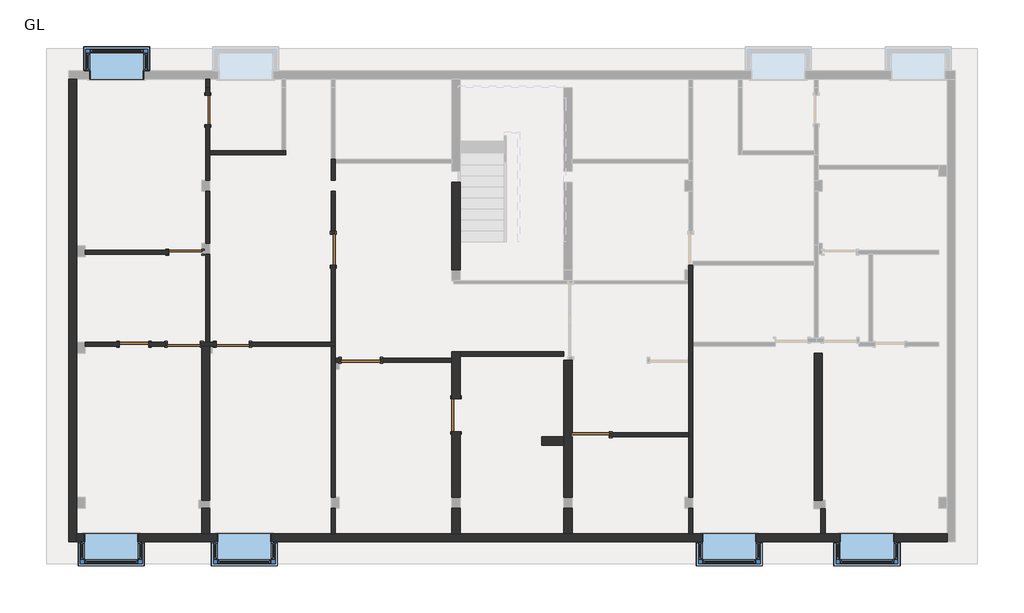
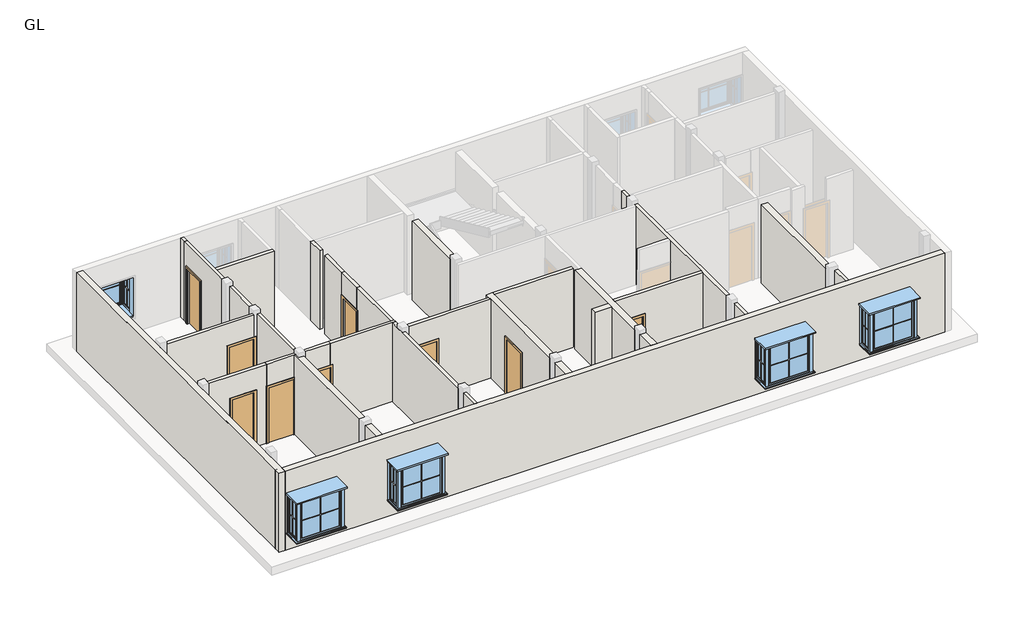
# One storey, part 1 of 3: 34 walls, 9 doors, 5 windows.
"""IFC4 building model written with IfcOpenShell, lengths in millimetres."""

from ifc_helpers import new_model, si_unit, frame, origin, place, context, project, spatial, polyline, outline, extrude, faceted_brep, transform, mapped, element, save
from components import m_door_single_panel_05506f71, m_door_single_panel_3722715f, door_07b5d71c, door_4c0a2014, door_82def9da, m_door_single_panel_3_x7_f8176753, m_door_single_panel_3_x7_ebb67e73, m_door_single_panel_3_x7_2af5d1b8, window_19bbd869

model = new_model("IFC4")

# Units and contexts
model_context = context("Model", 3, world=origin())
ifc_project = project(units=[si_unit("LENGTHUNIT", "METRE", prefix="MILLI")], contexts=[model_context])

# Site, building, storey
site = spatial("IfcSite", under=ifc_project)
building = spatial("IfcBuilding", under=site)
storey = spatial("IfcBuildingStorey", under=building, Name="GL", Elevation=3200.4)

# Doors
placement = place(None, origin())
m_door_single_panel_shape = m_door_single_panel_05506f71(model_context)
element("IfcDoor", 1, ObjectType="M_Door-Single-Panel", at=placement, inside=storey, context=model_context, shape_type="MappedRepresentation", body=[
    mapped(m_door_single_panel_shape, transform((1745.3012085, -1975.7432663, 3200.4), x_axis=(-1.0, 0.0, 0.0), y_axis=(0.0, -1.0, 0.0), z_axis=(0.0, 0.0, 1.0))),
])
m_door_single_panel_2_shape = m_door_single_panel_3722715f(model_context)
element("IfcDoor", 2, ObjectType="M_Door-Single-Panel", at=placement, inside=storey, context=model_context, shape_type="MappedRepresentation", body=[
    mapped(m_door_single_panel_2_shape, transform((-4598.3487995, 90.9578621, 3200.4), x_axis=(-1.0, 0.0, 0.0), y_axis=(0.0, -1.0, 0.0), z_axis=(0.0, 0.0, 1.0))),
])
door_shape = door_07b5d71c(model_context)
element("IfcDoor", 3, ObjectType="M_Door-Single-Panel : 2'10\"X7' 2", at=placement, inside=storey, context=model_context, shape_type="MappedRepresentation", body=[
    mapped(door_shape, transform((-5360.3487995, 3142.9626891, 3200.4), x_axis=(0.0, -1.0, 0.0), y_axis=(1.0, 0.0, 0.0), z_axis=(0.0, 0.0, 1.0))),
])
door_2_shape = door_4c0a2014(model_context)
element("IfcDoor", 4, ObjectType="M_Door-Single-Panel : 2'8\"X7'", at=placement, inside=storey, context=model_context, shape_type="MappedRepresentation", body=[
    mapped(door_2_shape, transform((-10873.4462614, 526.1567334, 3200.4), x_axis=(1.0, 0.0, 0.0), y_axis=(0.0, 1.0, 0.0), z_axis=(0.0, 0.0, 1.0))),
])
door_3_shape = door_82def9da(model_context)
element("IfcDoor", 5, ObjectType="M_Door-Single-Panel : 2'8\"X7'", at=placement, inside=storey, context=model_context, shape_type="MappedRepresentation", body=[
    mapped(door_3_shape, transform((-8827.4487992, 7008.6751452, 3200.4), x_axis=(0.0, 1.0, 0.0), y_axis=(-1.0, 0.0, 0.0), z_axis=(0.0, 0.0, 1.0))),
])
m_door_single_panel_3_x7_shape = m_door_single_panel_3_x7_f8176753(model_context)
element("IfcDoor", 6, ObjectType="M_Door-Single-Panel : 3'X7'", at=placement, inside=storey, context=model_context, shape_type="MappedRepresentation", body=[
    mapped(m_door_single_panel_3_x7_shape, transform((-9456.0987989, 3078.8567332, 3200.4), x_axis=(1.0, 0.0, 0.0), y_axis=(0.0, 1.0, 0.0), z_axis=(0.0, 0.0, 1.0))),
])
element("IfcDoor", 7, ObjectType="M_Door-Single-Panel : 3'X7'", at=placement, inside=storey, context=model_context, shape_type="MappedRepresentation", body=[
    mapped(m_door_single_panel_3_x7_shape, transform((-8144.8381465, 526.1567334, 3200.4), x_axis=(-1.0, 0.0, 0.0), y_axis=(0.0, -1.0, 0.0), z_axis=(0.0, 0.0, 1.0))),
])
m_door_single_panel_3_x7_2_shape = m_door_single_panel_3_x7_ebb67e73(model_context)
element("IfcDoor", 8, ObjectType="M_Door-Single-Panel : 3'X7'", at=placement, inside=storey, context=model_context, shape_type="MappedRepresentation", body=[
    mapped(m_door_single_panel_3_x7_2_shape, transform((-9494.1987992, 526.1567334, 3200.4), x_axis=(1.0, 0.0, 0.0), y_axis=(0.0, 1.0, 0.0), z_axis=(0.0, 0.0, 1.0))),
])
m_door_single_panel_3_x7_3_shape = m_door_single_panel_3_x7_2af5d1b8(model_context)
element("IfcDoor", 9, ObjectType="M_Door-Single-Panel : 3'X7'", at=placement, inside=storey, context=model_context, shape_type="MappedRepresentation", body=[
    mapped(m_door_single_panel_3_x7_3_shape, transform((-1963.0987998, -1433.0421379, 3200.4), x_axis=(0.0, -1.0, 0.0), y_axis=(1.0, 0.0, 0.0), z_axis=(0.0, 0.0, 1.0))),
])

# Walls
element("IfcWall", 10, ObjectType="4.5\"", at=placement, inside=storey, context=model_context, shape_type="SweptSolid", body=[
    extrude(outline(polyline([(2711.1626891, 6248.4), (3671.8272228, 6248.4), (3671.8272228, 3200.4), (3574.7626891, 3200.4), (3574.7626891, 5334.0), (2711.1626891, 5334.0), (2711.1626891, 6248.4)])), frame((-5417.4987995, 0.0, 0.0), z_axis=(1.0, 0.0, 0.0), x_axis=(0.0, 1.0, 0.0)), (0.0, 0.0, 1.0), 114.3),
])
element("IfcWall", 11, ObjectType="4.5\"", at=placement, inside=storey, context=model_context, shape_type="Brep", body=[
    faceted_brep([(-7690.1644155, 469.0067334, 6248.4), (-8713.148796, 469.0067334, 6248.4), (-8771.750543, 469.0067334, 6248.4), (-9000.350543, 469.0067334, 6248.4), (-10009.8462614, 469.0067334, 6248.4), (-10009.8462614, 469.0067334, 3200.4), (-9951.3987992, 469.0067334, 3200.4), (-9951.3987992, 469.0067334, 5334.0), (-9036.9987992, 469.0067334, 5334.0), (-9036.9987992, 469.0067334, 3200.4), (-9000.350543, 469.0067334, 3200.4), (-8771.750543, 469.0067334, 3200.4), (-8713.148796, 469.0067334, 3200.4), (-8602.0381465, 469.0067334, 3200.4), (-8602.0381465, 469.0067334, 5334.0), (-7690.1644155, 469.0067334, 5334.0), (-10009.8462614, 583.3067334, 6248.4), (-8941.748796, 583.3067334, 6248.4), (-8713.148796, 583.3067334, 6248.4), (-7690.1644155, 583.3067334, 6248.4), (-7690.1644155, 583.3067334, 5334.0), (-8602.0381465, 583.3067334, 5334.0), (-8602.0381465, 583.3067334, 3200.4), (-9036.9987992, 583.3067334, 3200.4), (-9036.9987992, 583.3067334, 5334.0), (-9951.3987992, 583.3067334, 5334.0), (-9951.3987992, 583.3067334, 3200.4), (-10009.8462614, 583.3067334, 3200.4)], [[[0, 1, 2, 3, 4, 5, 6, 7, 8, 9, 10, 11, 12, 13, 14, 15]], [[16, 17, 18, 19, 20, 21, 22, 23, 24, 25, 26, 27]], [[5, 27, 26, 6]], [[9, 23, 22, 13, 12, 11, 10]], [[19, 0, 15, 20]], [[4, 3, 2, 1, 0, 19, 18, 17, 16]], [[5, 4, 16, 27]], [[8, 24, 23, 9]], [[7, 25, 24, 8]], [[25, 7, 6, 26]], [[21, 14, 13, 22]], [[14, 21, 20, 15]]]),
])
element("IfcWall", 12, ObjectType="4.5\"", at=placement, inside=storey, context=model_context, shape_type="SweptSolid", body=[
    extrude(outline(polyline([(6248.4, 4475.8012082), (6248.4, 1250.0012085), (5334.0, 1250.0012085), (5334.0, 2278.7012085), (3200.4, 2278.7012085), (3200.4, 4475.8012082), (6248.4, 4475.8012082)])), frame((0.0, -2032.8932663, 0.0), z_axis=(0.0, 1.0, 0.0), x_axis=(0.0, 0.0, 1.0)), (0.0, 0.0, 1.0), 114.3),
])
element("IfcWall", 13, ObjectType="4.5\"", at=placement, inside=storey, context=model_context, shape_type="SweptSolid", body=[
    extrude(outline(polyline([(1021.4012085, 202.3067742), (-1848.7987998, 202.3067742), (-1848.7987998, 316.6067742), (1021.4012085, 316.6067742), (1021.4012085, 202.3067742)])), frame((0.0, 0.0, 3200.4), z_axis=(0.0, 0.0, 1.0), x_axis=(1.0, 0.0, 0.0)), (0.0, 0.0, 1.0), 3048.0),
])
element("IfcWall", 14, ObjectType="4.5\"", at=placement, inside=storey, context=model_context, shape_type="Brep", body=[
    faceted_brep([(-5417.4987995, 469.0067334, 3200.4), (-5417.4987995, -3709.2932193, 3200.4), (-5417.4987995, -3709.2932193, 6248.4), (-5417.4987995, -156.6921379, 6248.4), (-5417.4987995, 148.1078621, 6248.4), (-5417.4987995, 469.0067334, 6248.4), (-5303.1987995, 469.0067334, 3200.4), (-5303.1987995, 469.0067334, 6248.4), (-5303.1987995, 148.1078621, 6248.4), (-5303.1987995, 33.8078621, 6248.4), (-5303.1987995, -156.6921379, 6248.4), (-5303.1987995, -3709.2932193, 6248.4), (-5303.1987995, -3709.2932193, 3200.4), (-5303.1987995, -156.6921379, 3200.4), (-5303.1987995, 33.8078621, 3200.4), (-5303.1987995, 148.1078621, 3200.4)], [[[0, 1, 2, 3, 4, 5]], [[6, 7, 8, 9, 10, 11, 12, 13, 14, 15]], [[1, 0, 6, 15, 14, 13, 12]], [[2, 1, 12, 11]], [[5, 4, 3, 2, 11, 10, 9, 8, 7]], [[0, 5, 7, 6]]]),
])
element("IfcWall", 15, ObjectType="4.5\"", at=placement, inside=storey, context=model_context, shape_type="SweptSolid", body=[
    extrude(outline(polyline([(-5417.4987963, -4712.5932661), (-5417.4987963, -4014.0932193), (-5303.1987963, -4014.0932193), (-5303.1987963, -4712.5932661), (-5417.4987963, -4712.5932661)])), frame((0.0, 0.0, 3200.4), z_axis=(0.0, 0.0, 1.0), x_axis=(1.0, 0.0, 0.0)), (0.0, 0.0, 1.0), 3048.0),
])
element("IfcWall", 16, ObjectType="4.5\"", at=placement, inside=storey, context=model_context, shape_type="SweptSolid", body=[
    extrude(outline(polyline([(4475.8012082, -4712.5932661), (4475.8012082, -4014.0932193), (4590.1012082, -4014.0932193), (4590.1012082, -4712.5932661), (4475.8012082, -4712.5932661)])), frame((0.0, 0.0, 3200.4), z_axis=(0.0, 0.0, 1.0), x_axis=(1.0, 0.0, 0.0)), (0.0, 0.0, 1.0), 3048.0),
])
element("IfcWall", 17, ObjectType="4.5\"", at=placement, inside=storey, context=model_context, shape_type="SweptSolid", body=[
    extrude(outline(polyline([(8132.2646942, -4712.5932661), (8132.2646942, -4015.9914801), (8246.5646942, -4015.9914801), (8246.5646942, -4712.5932661), (8132.2646942, -4712.5932661)])), frame((0.0, 0.0, 3200.4), z_axis=(0.0, 0.0, 1.0), x_axis=(1.0, 0.0, 0.0)), (0.0, 0.0, 1.0), 3048.0),
])
element("IfcWall", 18, ObjectType="4.5\"", at=placement, inside=storey, context=model_context, shape_type="SweptSolid", body=[
    extrude(outline(polyline([(-8770.2987992, 7860.4067329), (-8770.2987992, 7631.8067329), (-8884.5987992, 7631.8067329), (-8884.5987992, 7860.4067329), (-8770.2987992, 7860.4067329)])), frame((0.0, 0.0, 3200.4), z_axis=(0.0, 0.0, 1.0), x_axis=(1.0, 0.0, 0.0)), (0.0, 0.0, 1.0), 3048.0),
])
element("IfcWall", 19, ObjectType="4.5\" 2", at=placement, inside=storey, context=model_context, shape_type="SweptSolid", body=[
    extrude(outline(polyline([(6248.4, -8998.8987989), (6248.4, -12224.6987989), (3200.4, -12224.6987989), (3200.4, -9913.2987989), (5334.0, -9913.2987989), (5334.0, -8998.8987989), (6248.4, -8998.8987989)])), frame((0.0, 3021.7067332, 0.0), z_axis=(0.0, 1.0, 0.0), x_axis=(0.0, 0.0, 1.0)), (0.0, 0.0, 1.0), 114.3),
])
element("IfcWall", 20, ObjectType="4.5\" 2", at=placement, inside=storey, context=model_context, shape_type="SweptSolid", body=[
    extrude(outline(polyline([(-8770.2987992, 4761.606733), (-8770.2987992, 3326.5067332), (-8884.5987992, 3326.5067332), (-8884.5987992, 4761.606733), (-8770.2987992, 4761.606733)])), frame((0.0, 0.0, 3200.4), z_axis=(0.0, 0.0, 1.0), x_axis=(1.0, 0.0, 0.0)), (0.0, 0.0, 1.0), 3048.0),
])
element("IfcWall", 21, ObjectType="4.5\" 2", at=placement, inside=storey, context=model_context, shape_type="Brep", body=[
    faceted_brep([(-8770.2987992, 7415.0751452, 5334.0), (-8770.2987992, 7415.0751452, 3200.4), (-8770.2987992, 7631.8067329, 3200.4), (-8770.2987992, 7631.8067329, 6248.4), (-8770.2987992, 5879.2067329, 6248.4), (-8770.2987992, 5764.9067329, 6248.4), (-8770.2987992, 5066.406733, 6248.4), (-8770.2987992, 5066.406733, 3200.4), (-8770.2987992, 5764.9067329, 3200.4), (-8770.2987992, 5879.2067329, 3200.4), (-8770.2987992, 6602.2751452, 3200.4), (-8770.2987992, 6602.2751452, 5334.0), (-8884.5987992, 7631.8067329, 3200.4), (-8884.5987992, 7415.0751452, 3200.4), (-8884.5987992, 7415.0751452, 5334.0), (-8884.5987992, 6602.2751452, 5334.0), (-8884.5987992, 6602.2751452, 3200.4), (-8884.5987992, 5066.406733, 3200.4), (-8884.5987992, 5066.406733, 6248.4), (-8884.5987992, 7631.8067329, 6248.4)], [[[0, 1, 2, 3, 4, 5, 6, 7, 8, 9, 10, 11]], [[12, 13, 14, 15, 16, 17, 18, 19]], [[2, 1, 13, 12]], [[10, 9, 8, 7, 17, 16]], [[3, 2, 12, 19]], [[6, 5, 4, 3, 19, 18]], [[7, 6, 18, 17]], [[14, 13, 1, 0]], [[15, 14, 0, 11]], [[16, 15, 11, 10]]]),
])
element("IfcWall", 22, ObjectType="4.5\" 2", at=placement, inside=storey, context=model_context, shape_type="Brep", body=[
    faceted_brep([(-8770.2987992, 5764.9067329, 3200.4), (-6674.7987994, 5764.9067329, 3200.4), (-6674.7987994, 5764.9067329, 6248.4), (-8770.2987992, 5764.9067329, 6248.4), (-8770.2987992, 5879.2067329, 3200.4), (-8770.2987992, 5879.2067329, 6248.4), (-6789.0987994, 5879.2067329, 6248.4), (-6674.7987994, 5879.2067329, 6248.4), (-6674.7987994, 5879.2067329, 3200.4), (-6789.0987994, 5879.2067329, 3200.4)], [[[0, 1, 2, 3]], [[4, 5, 6, 7, 8, 9]], [[1, 0, 4, 9, 8]], [[3, 2, 7, 6, 5]], [[0, 3, 5, 4]], [[2, 1, 8, 7]]]),
])
element("IfcWall", 23, ObjectType="4.5\" 2", at=placement, inside=storey, context=model_context, shape_type="SweptSolid", body=[
    extrude(outline(polyline([(5334.0, -10467.0462614), (3200.4, -10467.0462614), (3200.4, -10009.8462614), (6248.4, -10009.8462614), (6248.4, -12224.6987989), (3200.4, -12224.6987989), (3200.4, -11279.8462614), (5334.0, -11279.8462614), (5334.0, -10467.0462614)])), frame((0.0, 469.0067334, 0.0), z_axis=(0.0, 1.0, 0.0), x_axis=(0.0, 0.0, 1.0)), (0.0, 0.0, 1.0), 114.3),
])
element("IfcWall", 24, ObjectType="4.5\" 2", at=placement, inside=storey, context=model_context, shape_type="SweptSolid", body=[
    extrude(outline(polyline([(-8770.298796, 3021.7067332), (-8770.298796, 583.3067804), (-8884.598796, 583.3067804), (-8884.598796, 3021.7067332), (-8770.298796, 3021.7067332)])), frame((0.0, 0.0, 3200.4), z_axis=(0.0, 0.0, 1.0), x_axis=(1.0, 0.0, 0.0)), (0.0, 0.0, 1.0), 3048.0),
])
element("IfcWall", 25, ObjectType="4.5\" 2", at=placement, inside=storey, context=model_context, shape_type="Brep", body=[
    faceted_brep([(-5303.1987995, 469.0067334, 6248.4), (-5417.4987995, 469.0067334, 6248.4), (-7690.1644155, 469.0067334, 6248.4), (-7690.1644155, 469.0067334, 5334.0), (-7687.6381465, 469.0067334, 5334.0), (-7687.6381465, 469.0067334, 3200.4), (-5417.4987995, 469.0067334, 3200.4), (-5303.1987995, 469.0067334, 3200.4), (-7690.1644155, 583.3067334, 6248.4), (-5417.4987995, 583.3067334, 6248.4), (-5303.1987995, 583.3067334, 6248.4), (-5303.1987995, 583.3067334, 3200.4), (-5417.4987995, 583.3067334, 3200.4), (-7687.6381465, 583.3067334, 3200.4), (-7687.6381465, 583.3067334, 5334.0), (-7690.1644155, 583.3067334, 5334.0)], [[[0, 1, 2, 3, 4, 5, 6, 7]], [[8, 9, 10, 11, 12, 13, 14, 15]], [[11, 7, 6, 5, 13, 12]], [[2, 1, 0, 10, 9, 8]], [[2, 8, 15, 3]], [[0, 7, 11, 10]], [[14, 4, 3, 15]], [[4, 14, 13, 5]]]),
])
element("IfcWall", 26, ObjectType="4.5\" 2", at=placement, inside=storey, context=model_context, shape_type="SweptSolid", body=[
    extrude(outline(polyline([(-5303.1987995, 2709.1475436), (-5303.1987995, 583.3067334), (-5417.4987995, 583.3067334), (-5417.4987995, 2709.1475436), (-5303.1987995, 2709.1475436)])), frame((0.0, 0.0, 3200.4), z_axis=(0.0, 0.0, 1.0), x_axis=(1.0, 0.0, 0.0)), (0.0, 0.0, 1.0), 3048.0),
])
element("IfcWall", 27, ObjectType="4.5\" 2", at=placement, inside=storey, context=model_context, shape_type="Brep", body=[
    faceted_brep([(-5303.1987995, 2709.1475436, 3200.4), (-5303.1987995, 2711.1626891, 3200.4), (-5303.1987995, 2711.1626891, 5334.0), (-5303.1987995, 2711.1626891, 6248.4), (-5303.1987995, 2709.1475436, 6248.4), (-5417.4987995, 2709.1475436, 3200.4), (-5417.4987995, 2709.1475436, 6248.4), (-5417.4987995, 2711.1626891, 6248.4), (-5417.4987995, 2711.1626891, 5334.0), (-5417.4987995, 2711.1626891, 3200.4)], [[[0, 1, 2, 3, 4]], [[5, 6, 7, 8, 9]], [[1, 0, 5, 9]], [[3, 2, 1, 9, 8, 7]], [[4, 3, 7, 6]], [[0, 4, 6, 5]]]),
])
element("IfcWall", 28, ObjectType="4.5\" 2", at=placement, inside=storey, context=model_context, shape_type="SweptSolid", body=[
    extrude(outline(polyline([(-5303.1987995, 4761.606733), (-5303.1987995, 3671.8272228), (-5417.4987995, 3671.8272228), (-5417.4987995, 4761.606733), (-5303.1987995, 4761.606733)])), frame((0.0, 0.0, 3200.4), z_axis=(0.0, 0.0, 1.0), x_axis=(1.0, 0.0, 0.0)), (0.0, 0.0, 1.0), 3048.0),
])
element("IfcWall", 29, ObjectType="4.5\" 2", at=placement, inside=storey, context=model_context, shape_type="Brep", body=[
    faceted_brep([(-5303.1987995, 5066.406733, 3200.4), (-5303.1987995, 5536.3067329, 3200.4), (-5303.1987995, 5650.6067329, 3200.4), (-5303.1987995, 5650.6067329, 6248.4), (-5303.1987995, 5536.3067329, 6248.4), (-5303.1987995, 5066.406733, 6248.4), (-5417.4987995, 5066.406733, 3200.4), (-5417.4987995, 5066.406733, 6248.4), (-5417.4987995, 5650.6067329, 6248.4), (-5417.4987995, 5650.6067329, 3200.4)], [[[0, 1, 2, 3, 4, 5]], [[6, 7, 8, 9]], [[2, 1, 0, 6, 9]], [[5, 4, 3, 8, 7]], [[0, 5, 7, 6]], [[3, 2, 9, 8]]]),
])
element("IfcWall", 30, ObjectType="4.5\" 2", at=placement, inside=storey, context=model_context, shape_type="Brep", body=[
    faceted_brep([(4475.8012082, -3709.2932193, 3200.4), (4475.8012082, -3709.2932193, 6248.4), (4475.8012082, -2032.8932663, 6248.4), (4475.8012082, -1918.5932663, 6248.4), (4475.8012082, 33.8078621, 6248.4), (4475.8012082, 148.1078621, 6248.4), (4475.8012082, 2196.2067742, 6248.4), (4475.8012082, 2285.1067742, 6248.4), (4475.8012082, 2589.9067742, 6248.4), (4475.8012082, 3132.0737955, 6248.4), (4475.8012082, 3132.0737955, 5334.0), (4475.8012082, 2711.1626891, 5334.0), (4475.8012082, 2711.1626891, 3200.4), (4475.8012082, 2589.9067742, 3200.4), (4475.8012082, 2285.1067742, 3200.4), (4475.8012082, 2196.2067742, 3200.4), (4475.8012082, 148.1078621, 3200.4), (4475.8012082, 33.8078621, 3200.4), (4475.8012082, -1918.5932663, 3200.4), (4475.8012082, -2032.8932663, 3200.4), (4590.1012082, -3709.2932193, 6248.4), (4590.1012082, -3709.2932193, 3200.4), (4590.1012082, 469.0067334, 3200.4), (4590.1012082, 583.3067334, 3200.4), (4590.1012082, 2711.1626891, 3200.4), (4590.1012082, 2711.1626891, 5334.0), (4590.1012082, 3132.0737955, 5334.0), (4590.1012082, 3132.0737955, 6248.4), (4590.1012082, 2825.4626891, 6248.4), (4590.1012082, 2711.1626891, 6248.4), (4590.1012082, 2589.9067742, 6248.4), (4590.1012082, 2285.1067742, 6248.4), (4590.1012082, 583.3067334, 6248.4), (4590.1012082, 469.0067334, 6248.4)], [[[0, 1, 2, 3, 4, 5, 6, 7, 8, 9, 10, 11, 12, 13, 14, 15, 16, 17, 18, 19]], [[20, 21, 22, 23, 24, 25, 26, 27, 28, 29, 30, 31, 32, 33]], [[21, 0, 19, 18, 17, 16, 15, 14, 13, 12, 24, 23, 22]], [[1, 0, 21, 20]], [[9, 8, 7, 6, 5, 4, 3, 2, 1, 20, 33, 32, 31, 30, 29, 28, 27]], [[9, 27, 26, 10]], [[11, 25, 24, 12]], [[25, 11, 10, 26]]]),
])
element("IfcWall", 31, ObjectType="4.5\" 2", at=placement, inside=storey, context=model_context, shape_type="Brep", body=[
    faceted_brep([(-5303.1987995, 33.8078621, 3200.4), (-5188.8987995, 33.8078621, 3200.4), (-5131.7487995, 33.8078621, 3200.4), (-5131.7487995, 33.8078621, 5334.0), (-4064.9487995, 33.8078621, 5334.0), (-4064.9487995, 33.8078621, 3200.4), (-2077.3987998, 33.8078621, 3200.4), (-2077.3987998, 33.8078621, 6248.4), (-5188.8987995, 33.8078621, 6248.4), (-5303.1987995, 33.8078621, 6248.4), (-5131.7487995, 148.1078621, 5334.0), (-5131.7487995, 148.1078621, 3200.4), (-5303.1987995, 148.1078621, 3200.4), (-5303.1987995, 148.1078621, 6248.4), (-5188.8987995, 148.1078621, 6248.4), (-2077.3987998, 148.1078621, 6248.4), (-2077.3987998, 148.1078621, 3200.4), (-4064.9487995, 148.1078621, 3200.4), (-4064.9487995, 148.1078621, 5334.0)], [[[0, 1, 2, 3, 4, 5, 6, 7, 8, 9]], [[10, 11, 12, 13, 14, 15, 16, 17, 18]], [[17, 16, 6, 5]], [[12, 11, 2, 1, 0]], [[9, 8, 7, 15, 14, 13]], [[7, 6, 16, 15]], [[0, 9, 13, 12]], [[3, 2, 11, 10]], [[4, 3, 10, 18]], [[5, 4, 18, 17]]]),
])
element("IfcWall", 32, ObjectType="9\"", at=placement, inside=storey, context=model_context, shape_type="Brep", body=[
    faceted_brep([(-12453.2987957, -4941.1932661, 3200.4), (-12453.2987957, -4712.5932661, 3200.4), (-12453.2987957, -4014.0932671, 3200.4), (-12453.2987957, -3709.2932671, 3200.4), (-12453.2987957, 278.5067334, 3200.4), (-12453.2987957, 583.3067334, 3200.4), (-12453.2987957, 2951.8567332, 3200.4), (-12453.2987957, 3256.6567332, 3200.4), (-12453.2987957, 7860.4067329, 3200.4), (-12453.2987957, 7860.4067329, 6248.4), (-12453.2987957, -4712.5932661, 6248.4), (-12453.2987957, -4941.1932661, 6248.4), (-12681.8987957, -4941.1932661, 3200.4), (-12681.8987957, -4941.1932661, 6248.4), (-12681.8987957, 7860.4067329, 6248.4), (-12681.8987957, 7860.4067329, 3200.4)], [[[0, 1, 2, 3, 4, 5, 6, 7, 8, 9, 10, 11]], [[12, 13, 14, 15]], [[8, 7, 6, 5, 4, 3, 2, 1, 0, 12, 15]], [[11, 10, 9, 14, 13]], [[9, 8, 15, 14]], [[0, 11, 13, 12]]]),
])
element("IfcWall", 33, ObjectType="9\"", at=placement, inside=storey, context=model_context, shape_type="Brep", body=[
    faceted_brep([(-12453.2987957, -4712.5932661, 3200.4), (-12453.2987957, -4014.0932671, 3200.4), (-12453.2987957, -3709.2932671, 3200.4), (-12453.2987957, 278.5067334, 3200.4), (-12453.2987957, 583.3067334, 3200.4), (-12453.2987957, 2951.8567332, 3200.4), (-12453.2987957, 3256.6567332, 3200.4), (-12453.2987957, 7860.4067329, 3200.4), (-12453.2987957, 7860.4067329, 6248.4), (-12453.2987957, -4712.5932661, 6248.4), (-12681.8987957, -4712.5932661, 3200.4), (-12681.8987957, -4712.5932661, 6248.4), (-12681.8987957, 7860.4067329, 6248.4), (-12681.8987957, 7860.4067329, 3200.4)], [[[0, 1, 2, 3, 4, 5, 6, 7, 8, 9]], [[10, 11, 12, 13]], [[7, 6, 5, 4, 3, 2, 1, 0, 10, 13]], [[9, 8, 12, 11]], [[8, 7, 13, 12]], [[0, 9, 11, 10]]]),
])
element("IfcWall", 34, ObjectType="9\"", at=placement, inside=storey, context=model_context, shape_type="Brep", body=[
    faceted_brep([(-9000.350543, 469.0067334, 3200.4), (-9000.350543, -3785.4932196, 3200.4), (-9000.350543, -3785.4932196, 6248.4), (-9000.350543, 469.0067334, 6248.4), (-8771.750543, 469.0067334, 3200.4), (-8771.750543, 469.0067334, 6248.4), (-8771.750543, 278.5067334, 6248.4), (-8771.750543, -3785.4932196, 6248.4), (-8771.750543, -3785.4932196, 3200.4), (-8771.750543, 278.5067334, 3200.4)], [[[0, 1, 2, 3]], [[4, 5, 6, 7, 8, 9]], [[1, 0, 4, 9, 8]], [[2, 1, 8, 7]], [[3, 2, 7, 6, 5]], [[0, 3, 5, 4]]]),
])
element("IfcWall", 35, ObjectType="9\"", at=placement, inside=storey, context=model_context, shape_type="Brep", body=[
    faceted_brep([(-2077.3987998, -1890.2421379, 5334.0), (-2077.3987998, -1890.2421379, 3200.4), (-2077.3987998, -3709.2932663, 3200.4), (-2077.3987998, -3709.2932663, 6248.4), (-2077.3987998, 33.8078621, 6248.4), (-2077.3987998, 148.1078621, 6248.4), (-2077.3987998, 316.6067742, 6248.4), (-2077.3987998, 316.6067742, 3200.4), (-2077.3987998, 148.1078621, 3200.4), (-2077.3987998, 33.8078621, 3200.4), (-2077.3987998, -975.8421379, 3200.4), (-2077.3987998, -975.8421379, 5334.0), (-1848.7987998, -3709.2932663, 3200.4), (-1848.7987998, -1890.2421379, 3200.4), (-1848.7987998, -1890.2421379, 5334.0), (-1848.7987998, -975.8421379, 5334.0), (-1848.7987998, -975.8421379, 3200.4), (-1848.7987998, 202.3067742, 3200.4), (-1848.7987998, 316.6067742, 3200.4), (-1848.7987998, 316.6067742, 6248.4), (-1848.7987998, 202.3067742, 6248.4), (-1848.7987998, -3709.2932663, 6248.4)], [[[0, 1, 2, 3, 4, 5, 6, 7, 8, 9, 10, 11]], [[12, 13, 14, 15, 16, 17, 18, 19, 20, 21]], [[2, 1, 13, 12]], [[10, 9, 8, 7, 18, 17, 16]], [[3, 2, 12, 21]], [[6, 5, 4, 3, 21, 20, 19]], [[7, 6, 19, 18]], [[14, 13, 1, 0]], [[15, 14, 0, 11]], [[16, 15, 11, 10]]]),
])
element("IfcWall", 36, ObjectType="9\"", at=placement, inside=storey, context=model_context, shape_type="SweptSolid", body=[
    extrude(outline(polyline([(1021.4012085, -2261.4932663), (412.152227, -2261.4932663), (412.152227, -2032.8932663), (1021.4012085, -2032.8932663), (1021.4012085, -2261.4932663)])), frame((0.0, 0.0, 3200.4), z_axis=(0.0, 0.0, 1.0), x_axis=(1.0, 0.0, 0.0)), (0.0, 0.0, 1.0), 3048.0),
])
element("IfcWall", 37, ObjectType="9\"", at=placement, inside=storey, context=model_context, shape_type="Brep", body=[
    faceted_brep([(1021.4012085, 90.9578621, 3200.4), (1021.4012085, -2032.8932663, 3200.4), (1021.4012085, -2261.4932663, 3200.4), (1021.4012085, -3709.2932193, 3200.4), (1021.4012085, -3709.2932193, 6248.4), (1021.4012085, -2261.4932663, 6248.4), (1021.4012085, -2032.8932663, 6248.4), (1021.4012085, 90.9578621, 6248.4), (1250.0012085, -3709.2932193, 6248.4), (1250.0012085, -3709.2932193, 3200.4), (1250.0012085, -2032.8932663, 3200.4), (1250.0012085, -2032.8932663, 5334.0), (1250.0012085, -1918.5932663, 5334.0), (1250.0012085, -1918.5932663, 3200.4), (1250.0012085, 90.9578621, 3200.4), (1250.0012085, 90.9578621, 6248.4), (1250.0012085, -1918.5932663, 6248.4), (1250.0012085, -2032.8932663, 6248.4), (1158.0082462, 90.9578621, 3200.4), (1211.9012085, -1918.5932663, 3200.4), (1211.9012085, -2032.8932663, 3200.4), (1158.0082462, 90.9578621, 6248.4), (1211.9012085, -1918.5932663, 5334.0), (1211.9012085, -2032.8932663, 5334.0)], [[[0, 1, 2, 3, 4, 5, 6, 7]], [[8, 9, 10, 11, 12, 13, 14, 15, 16, 17]], [[3, 2, 1, 0, 18, 14, 13, 19, 20, 10, 9]], [[4, 3, 9, 8]], [[7, 6, 5, 4, 8, 17, 16, 15, 21]], [[0, 7, 21, 15, 14, 18]], [[22, 19, 13, 12]], [[20, 23, 11, 10]], [[19, 22, 23, 20]], [[23, 22, 12, 11]]]),
])
element("IfcWall", 38, ObjectType="9\"", at=placement, inside=storey, context=model_context, shape_type="SweptSolid", body=[
    extrude(outline(polyline([(-2074.1417538, 2589.906774), (-2074.1417538, 5015.606774), (-1845.5417538, 5015.606774), (-1845.5417538, 2589.906774), (-2074.1417538, 2589.906774)])), frame((0.0, 0.0, 3200.4), z_axis=(0.0, 0.0, 1.0), x_axis=(1.0, 0.0, 0.0)), (0.0, 0.0, 1.0), 3048.0),
])
element("IfcWall", 39, ObjectType="9\"", at=placement, inside=storey, context=model_context, shape_type="SweptSolid", body=[
    extrude(outline(polyline([(7942.9012047, -3785.4932666), (7942.9012047, 278.5067334), (8171.5012047, 278.5067334), (8171.5012047, -3785.4932666), (7942.9012047, -3785.4932666)])), frame((0.0, 0.0, 3200.4), z_axis=(0.0, 0.0, 1.0), x_axis=(1.0, 0.0, 0.0)), (0.0, 0.0, 1.0), 3048.0),
])
element("IfcWall", 40, ObjectType="9\" 2", at=placement, inside=storey, context=model_context, shape_type="Brep", body=[
    faceted_brep([(-12453.2987957, -4941.1932661, 3200.4), (11625.9012075, -4941.1932662, 3200.4), (11625.9012075, -4941.1932662, 6248.4), (-12453.2987957, -4941.1932661, 6248.4), (-12250.7987957, -4941.1932661, 5351.2), (-10750.7987957, -4941.1932661, 5351.2), (-10750.7987957, -4941.1932661, 3800.4), (-12250.7987957, -4941.1932661, 3800.4), (-8569.250543, -4941.1932661, 5351.2), (-7069.250543, -4941.1932661, 5351.2), (-7069.250543, -4941.1932661, 3800.4), (-8569.250543, -4941.1932661, 3800.4), (4849.7512082, -4941.1932661, 5351.2), (6349.7512082, -4941.1932661, 5351.2), (6349.7512082, -4941.1932661, 3800.4), (4849.7512082, -4941.1932661, 3800.4), (8658.6146942, -4941.1932661, 5351.2), (10158.6146942, -4941.1932661, 5351.2), (10158.6146942, -4941.1932661, 3800.4), (8658.6146942, -4941.1932661, 3800.4), (-12453.2987957, -4712.5932661, 3200.4), (-12453.2987957, -4712.5932661, 6248.4), (-9000.350543, -4712.5932661, 6248.4), (-8771.750543, -4712.5932661, 6248.4), (-5417.4987963, -4712.5932661, 6248.4), (-5303.1987963, -4712.5932661, 6248.4), (-2077.3987998, -4712.5932661, 6248.4), (-1848.7987998, -4712.5932661, 6248.4), (1021.4012085, -4712.5932661, 6248.4), (1250.0012085, -4712.5932661, 6248.4), (4475.8012082, -4712.5932661, 6248.4), (4590.1012082, -4712.5932661, 6248.4), (8132.2646942, -4712.5932661, 6248.4), (8246.5646942, -4712.5932661, 6248.4), (11625.9012075, -4712.5932662, 6248.4), (11625.9012075, -4712.5932662, 3200.4), (8246.5646942, -4712.5932661, 3200.4), (8132.2646942, -4712.5932661, 3200.4), (4590.1012082, -4712.5932661, 3200.4), (4475.8012082, -4712.5932661, 3200.4), (1250.0012085, -4712.5932661, 3200.4), (1021.4012085, -4712.5932661, 3200.4), (-1848.7987998, -4712.5932661, 3200.4), (-2077.3987998, -4712.5932661, 3200.4), (-5303.1987963, -4712.5932661, 3200.4), (-5417.4987963, -4712.5932661, 3200.4), (-8771.750543, -4712.5932661, 3200.4), (-9000.350543, -4712.5932661, 3200.4), (-12250.7987957, -4712.5932661, 5351.2), (-12250.7987957, -4712.5932661, 3800.4), (-10750.7987957, -4712.5932661, 3800.4), (-10750.7987957, -4712.5932661, 5351.2), (-8569.250543, -4712.5932661, 5351.2), (-8569.250543, -4712.5932661, 3800.4), (-7069.250543, -4712.5932661, 3800.4), (-7069.250543, -4712.5932661, 5351.2), (4849.7512082, -4712.5932661, 5351.2), (4849.7512082, -4712.5932661, 3800.4), (6349.7512082, -4712.5932661, 3800.4), (6349.7512082, -4712.5932661, 5351.2), (8658.6146942, -4712.5932661, 5351.2), (8658.6146942, -4712.5932661, 3800.4), (10158.6146942, -4712.5932661, 3800.4), (10158.6146942, -4712.5932661, 5351.2)], [[[0, 1, 2, 3], [4, 5, 6, 7], [8, 9, 10, 11], [12, 13, 14, 15], [16, 17, 18, 19]], [[20, 21, 22, 23, 24, 25, 26, 27, 28, 29, 30, 31, 32, 33, 34, 35, 36, 37, 38, 39, 40, 41, 42, 43, 44, 45, 46, 47], [48, 49, 50, 51], [52, 53, 54, 55], [56, 57, 58, 59], [60, 61, 62, 63]], [[1, 0, 20, 47, 46, 45, 44, 43, 42, 41, 40, 39, 38, 37, 36, 35]], [[3, 2, 34, 33, 32, 31, 30, 29, 28, 27, 26, 25, 24, 23, 22, 21]], [[2, 1, 35, 34]], [[0, 3, 21, 20]], [[49, 48, 4, 7]], [[50, 49, 7, 6]], [[51, 50, 6, 5]], [[48, 51, 5, 4]], [[53, 52, 8, 11]], [[54, 53, 11, 10]], [[55, 54, 10, 9]], [[52, 55, 9, 8]], [[57, 56, 12, 15]], [[58, 57, 15, 14]], [[59, 58, 14, 13]], [[56, 59, 13, 12]], [[61, 60, 16, 19]], [[62, 61, 19, 18]], [[63, 62, 18, 17]], [[60, 63, 17, 16]]]),
])
element("IfcWall", 41, ObjectType="9\" 2", at=placement, inside=storey, context=model_context, shape_type="SweptSolid", body=[
    extrude(outline(polyline([(-9000.350543, -4712.5932661), (-9000.350543, -4014.0932196), (-8771.750543, -4014.0932196), (-8771.750543, -4712.5932661), (-9000.350543, -4712.5932661)])), frame((0.0, 0.0, 3200.4), z_axis=(0.0, 0.0, 1.0), x_axis=(1.0, 0.0, 0.0)), (0.0, 0.0, 1.0), 3048.0),
])
element("IfcWall", 42, ObjectType="9\" 2", at=placement, inside=storey, context=model_context, shape_type="SweptSolid", body=[
    extrude(outline(polyline([(-2077.3987998, -4712.5932661), (-2077.3987998, -4014.0932663), (-1848.7987998, -4014.0932663), (-1848.7987998, -4712.5932661), (-2077.3987998, -4712.5932661)])), frame((0.0, 0.0, 3200.4), z_axis=(0.0, 0.0, 1.0), x_axis=(1.0, 0.0, 0.0)), (0.0, 0.0, 1.0), 3048.0),
])
element("IfcWall", 43, ObjectType="9\" 2", at=placement, inside=storey, context=model_context, shape_type="SweptSolid", body=[
    extrude(outline(polyline([(1021.4012085, -4712.5932661), (1021.4012085, -4014.0932193), (1250.0012085, -4014.0932193), (1250.0012085, -4712.5932661), (1021.4012085, -4712.5932661)])), frame((0.0, 0.0, 3200.4), z_axis=(0.0, 0.0, 1.0), x_axis=(1.0, 0.0, 0.0)), (0.0, 0.0, 1.0), 3048.0),
])

# Windows
window_shape = window_19bbd869(model_context)
element("IfcWindow", 44, ObjectType="4'.8\"x3'.8\"", at=placement, inside=storey, context=model_context, shape_type="MappedRepresentation", body=[
    mapped(window_shape, transform((-11500.7987957, -4826.8932661, 3200.4), x_axis=(-1.0, 0.0, 0.0), y_axis=(0.0, -1.0, 0.0), z_axis=(0.0, 0.0, 1.0))),
])
element("IfcWindow", 45, ObjectType="4'.8\"x3'.8\"", at=placement, inside=storey, context=model_context, shape_type="MappedRepresentation", body=[
    mapped(window_shape, transform((-7819.250543, -4826.8932661, 3200.4), x_axis=(-1.0, 0.0, 0.0), y_axis=(0.0, -1.0, 0.0), z_axis=(0.0, 0.0, 1.0))),
])
element("IfcWindow", 46, ObjectType="4'.8\"x3'.8\"", at=placement, inside=storey, context=model_context, shape_type="MappedRepresentation", body=[
    mapped(window_shape, transform((5599.7512082, -4826.8932661, 3200.4), x_axis=(-1.0, 0.0, 0.0), y_axis=(0.0, -1.0, 0.0), z_axis=(0.0, 0.0, 1.0))),
])
element("IfcWindow", 47, ObjectType="4'.8\"x3'.8\"", at=placement, inside=storey, context=model_context, shape_type="MappedRepresentation", body=[
    mapped(window_shape, transform((9408.6146942, -4826.8932661, 3200.4), x_axis=(-1.0, 0.0, 0.0), y_axis=(0.0, -1.0, 0.0), z_axis=(0.0, 0.0, 1.0))),
])
element("IfcWindow", 48, ObjectType="4'.8\"x3'.8\"", at=placement, inside=storey, context=model_context, shape_type="MappedRepresentation", body=[
    mapped(window_shape, transform((-11348.3987957, 7974.7067329, 3200.4), x_axis=(1.0, 0.0, 0.0), y_axis=(0.0, 1.0, 0.0), z_axis=(0.0, 0.0, 1.0))),
])

save(model, "model.ifc")

# Revit data of these elements
# Type "M_Door-Single-Panel"
#   Type Mark = "14"
#   Construction Type Id = "DOOR"
#   Assembly Code = "C1020300"
#   Analytic Construction = "Wooden"
#   Thickness = 0' - 1.9685"
#   Thermal Resistance (R) = 2.5876 (h·ft²·°F)/BTU
#   Swing Angle [instance default] = 90.00°
#   Heat Transfer Coefficient (U) = 0.3865 BTU/(h·ft²·°F)
#   Height = 7' - 0"
#   Trim Projection Ext = 0' - 0.98425"
#   Trim Projection Int = 0' - 0.98425"
#   Trim Width = 0' - 3.14961"
#   Width = 3' - 6"
#   Define Thermal Properties by = 1
#   Panel Material = Wood - Birch - Solid Stained Light Low Gloss
#   Trim Material = Paint - Sienna
#   Visual Light Transmittance = 0
#   Solar Heat Gain Coefficient = 0
#   Function = (empty or 0)
#   Wall Closure = (empty or 0)
# Type "M_Door-Single-Panel : 2'10\"X7' 2"
#   Type Mark = "10"
#   Construction Type Id = "DOOR"
#   Assembly Code = "C1020300"
#   Analytic Construction = "Wooden"
#   Thickness = 0' - 1.9685"
#   Thermal Resistance (R) = 2.5876 (h·ft²·°F)/BTU
#   Swing Angle [instance default] = 90.00°
#   Heat Transfer Coefficient (U) = 0.3865 BTU/(h·ft²·°F)
#   Height = 7' - 0"
#   Trim Projection Ext = 0' - 0.98425"
#   Trim Projection Int = 0' - 0.98425"
#   Trim Width = 0' - 3.14961"
#   Width = 2' - 10"
#   Define Thermal Properties by = 1
#   Panel Material = Wood - Birch - Solid Stained Light Low Gloss
#   Trim Material = Paint - Sienna
#   Visual Light Transmittance = 0
#   Solar Heat Gain Coefficient = 0
#   Function = (empty or 0)
#   Wall Closure = (empty or 0)
# Type "M_Door-Single-Panel : 2'8\"X7'"
#   Type Mark = "9"
#   Construction Type Id = "DOOR"
#   Assembly Code = "C1020300"
#   Analytic Construction = "Wooden"
#   Thickness = 0' - 1.9685"
#   Thermal Resistance (R) = 2.5876 (h·ft²·°F)/BTU
#   Swing Angle [instance default] = 90.00°
#   Heat Transfer Coefficient (U) = 0.3865 BTU/(h·ft²·°F)
#   Height = 7' - 0"
#   Trim Projection Ext = 0' - 0.98425"
#   Trim Projection Int = 0' - 0.98425"
#   Trim Width = 0' - 3.14961"
#   Width = 2' - 8"
#   Define Thermal Properties by = 1
#   Panel Material = Wood - Birch - Solid Stained Light Low Gloss
#   Trim Material = Paint - Sienna
#   Visual Light Transmittance = 0
#   Solar Heat Gain Coefficient = 0
#   Function = (empty or 0)
#   Wall Closure = (empty or 0)
# Type "M_Door-Single-Panel : 3'X7'"
#   Type Mark = "11"
#   Construction Type Id = "DOOR"
#   Assembly Code = "C1020300"
#   Analytic Construction = "Wooden"
#   Thickness = 0' - 1.9685"
#   Thermal Resistance (R) = 2.5876 (h·ft²·°F)/BTU
#   Swing Angle [instance default] = 90.00°
#   Heat Transfer Coefficient (U) = 0.3865 BTU/(h·ft²·°F)
#   Height = 7' - 0"
#   Trim Projection Ext = 0' - 0.98425"
#   Trim Projection Int = 0' - 0.98425"
#   Trim Width = 0' - 3.14961"
#   Width = 3' - 0"
#   Define Thermal Properties by = 1
#   Panel Material = Wood - Birch - Solid Stained Light Low Gloss
#   Trim Material = Paint - Sienna
#   Visual Light Transmittance = 0
#   Solar Heat Gain Coefficient = 0
#   Function = (empty or 0)
#   Wall Closure = (empty or 0)
# Type "4.5\""
#   Assembly Code = "B2010"
#   Layers, outside or top first: 0' - 4 1/2" no material (function 1)
# Type "4.5\" 2"
#   Assembly Code = "B2010"
#   Layers, outside or top first: 0' - 4 1/2" no material (function 1)
# Type "9\""
#   Assembly Code = "B2010"
#   Layers, outside or top first: 0' - 9" no material (function 1)
# Type "9\" 2"
#   Assembly Code = "B2010"
#   Layers, outside or top first: 0' - 9" no material (function 1)
# Type "4'.8\"x3'.8\""
#   Type Mark = "20"
#   Fire Rating = "0.5h"
#   Assembly Code = "B2020100"
#   Analytic Construction = "1/8 in Pilkington single glazing"
#   Width = 4' - 11.05512"
#   Wall Thickness [instance default] = 0' - 5.90551"
#   Visual Light Transmittance = 0.9
#   Trim Width = 5' - 7.05512"
#   Trim Height = 4' - 11.05512"
#   Thermal Resistance (R) = 1.5394 (h·ft²·°F)/BTU
#   Solar Heat Gain Coefficient = 0.86
#   Rough Width = 4' - 11.64567"
#   Rough Height = 4' - 11.64567"
#   Height 1 = 5' - 1.05512"
#   Height = 4' - 11.05512"
#   Heat Transfer Coefficient (U) = 0.6496 BTU/(h·ft²·°F)
#   Depth = 1' - 11.62205"
#   Default Sill Height = 1' - 11.62205"
#   Side Muntin Visibility = yes
#   Center Muntin Visibility = yes
#   Interior Trim Visibility [instance default] = yes
#   Exterior Trim Visibility [instance default] = yes
#   Side Muntin Pattern = M_Muntin Pattern_2x2 : M_Muntin Pattern_2x2
#   Center Muntin Pattern = M_Muntin Pattern_2x2 : M_Muntin Pattern_2x2
#   Interior Trim Material = Wood - Stained
#   Exterior Trim Material = Clad - White
#   Exterior Trim = element 422966
#   Interior Trim = M_Trim-Window-Interior-Flat : Picture Frame
#   Interior Frame Material = Wood - Stained
#   Glass Panel Material = Glass
#   Exterior Frame Material = Clad - White
#   Wall Closure = (empty or 0)
# Elements 1, 2 (IfcDoor, "M_Door-Single-Panel")
#   Swing Angle = 90.00°
#   Phase Created = New Construction
#   Materials on its faces: "Paint - Sienna", "Wood - Birch - Solid Stained Light Low Gloss"
# Element 3 (IfcDoor, "M_Door-Single-Panel : 2'10\"X7' 2")
#   Swing Angle = 90.00°
#   Phase Created = New Construction
#   Materials on its faces: "Paint - Sienna", "Wood - Birch - Solid Stained Light Low Gloss"
# Elements 4, 5 (IfcDoor, "M_Door-Single-Panel : 2'8\"X7'")
#   Swing Angle = 90.00°
#   Phase Created = New Construction
#   Materials on its faces: "Paint - Sienna", "Wood - Birch - Solid Stained Light Low Gloss"
# Elements 6, 7, 8, 9 (IfcDoor, "M_Door-Single-Panel : 3'X7'")
#   Swing Angle = 90.00°
#   Phase Created = New Construction
#   Materials on its faces: "Paint - Sienna", "Wood - Birch - Solid Stained Light Low Gloss"
# Elements 10, 11, 12, 13, 14, 15, 16, 17, 18 (IfcWall, "4.5\"")
#   Top Offset = -0' - 6"
#   Base Offset = 0' - 0"
#   wall height = 10' - 0"
#   Phase Created = New Construction
#   Base Constraint = GL
#   Materials on its faces: "Default Wall"
# Elements 19, 20, 21, 22, 23, 24, 25, 26, 27, 28, 29, 30, 31 (IfcWall, "4.5\" 2")
#   Top Offset = -0' - 6"
#   Base Offset = 0' - 0"
#   wall height = 10' - 0"
#   Phase Created = New Construction
#   Base Constraint = GL
#   Materials on its faces: "Default Wall"
# Elements 32, 33, 34, 35, 36, 37, 38, 39 (IfcWall, "9\"")
#   Top Offset = -0' - 6"
#   Base Offset = 0' - 0"
#   wall height = 10' - 0"
#   Phase Created = New Construction
#   Base Constraint = GL
#   Materials on its faces: "Default Wall"
# Elements 40, 41, 42, 43 (IfcWall, "9\" 2")
#   Top Offset = -0' - 6"
#   Base Offset = 0' - 0"
#   wall height = 10' - 0"
#   Phase Created = New Construction
#   Base Constraint = GL
#   Materials on its faces: "Default Wall"
# Element 44 (IfcWindow, "4'.8\"x3'.8\"")
#   Mark = "227"
#   Interior Trim Visibility = yes
#   Exterior Trim Visibility = yes
#   Phase Created = New Construction
#   Materials on its faces: "Clad - White", "Wood - Stained", "Glass"
# Element 45 (IfcWindow, "4'.8\"x3'.8\"")
#   Mark = "228"
#   Interior Trim Visibility = yes
#   Exterior Trim Visibility = yes
#   Phase Created = New Construction
#   Materials on its faces: "Clad - White", "Wood - Stained", "Glass"
# Element 46 (IfcWindow, "4'.8\"x3'.8\"")
#   Mark = "229"
#   Interior Trim Visibility = yes
#   Exterior Trim Visibility = yes
#   Phase Created = New Construction
#   Materials on its faces: "Clad - White", "Wood - Stained", "Glass"
# Element 47 (IfcWindow, "4'.8\"x3'.8\"")
#   Mark = "230"
#   Interior Trim Visibility = yes
#   Exterior Trim Visibility = yes
#   Phase Created = New Construction
#   Materials on its faces: "Clad - White", "Wood - Stained", "Glass"
# Element 48 (IfcWindow, "4'.8\"x3'.8\"")
#   Mark = "271"
#   Interior Trim Visibility = yes
#   Exterior Trim Visibility = yes
#   Phase Created = New Construction
#   Materials on its faces: "Clad - White", "Wood - Stained", "Glass"
# Materials
#   "Wood - Birch - Solid Stained Light Low Gloss": class "Wood", colour RGB 210 159 95, transparency 0, Cost = 0
#   "Paint - Sienna": colour RGB 118 70 51, transparency 0, Cost = 0
#   "Wood - Stained": class "Wood", colour RGB 224 178 126, transparency 0, Cost = 0
#   "Clad - White": class "Wood", colour RGB 242 242 238, transparency 0, Cost = 0
#   "Glass": class "Glass", colour RGB 0 128 192, transparency 0.75, Description = "Soda Lime Glass", Cost = 0
#   "Default Wall": colour RGB 128 128 128, transparency 0, Cost = 0
